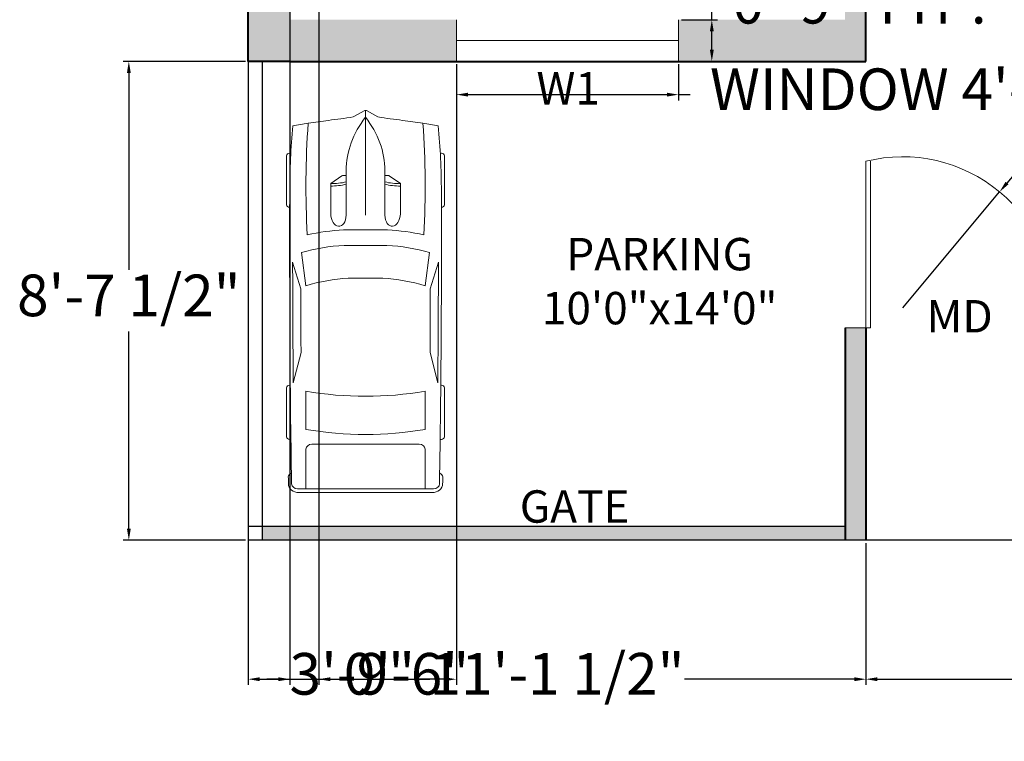
# Model space of a CAD drawing. Units: inches. Extents: x 1883 to 2353, y 1976 to 2541.
# Tile 1 of 5: x 1957 to 2170, y 1976 to 2132. Entities that reach past the tile are written whole.
import ezdxf

# ---------------------------------------------------------------- set-up
doc = ezdxf.new("R2010")
doc.units = ezdxf.units.IN
for name, color, linetype, lineweight in [('A-ANNO-DIMS', 2, 'Continuous', 18), ('A-ANNO-TEXT', 7, 'Continuous', 18), ('A-AREA-IDEN', 7, 'Continuous', 18), ('A-DOOR', 3, 'Continuous', 18), ('A-GLAZ', 4, 'Continuous', 18), ('A-WALL', 7, 'Continuous', 40), ('C-PRKG-VEHI', 8, 'Continuous', 13), ('C-SITE', 7, 'Continuous', 25)]:
    doc.layers.add(name, color=color, linetype=linetype, lineweight=lineweight)
doc.layers.add('A-WALL-PATT', color=67, linetype='Continuous', lineweight=13, true_color=0x727430)
doc.layers.add('C-SITE-PATT', color=18, linetype='Continuous', lineweight=13, true_color=0x000000)
doc.styles.get("Standard").update_dxf_attribs({"font": 'arial.ttf'})
doc.dimstyles.new('ISO-25', dxfattribs={"dimtxt": 9, "dimasz": 2.5, "dimexe": 1.25, "dimexo": 0.625, "dimgap": 2, "dimtad": 0, "dimtih": 1, "dimtoh": 1, "dimdec": 1, "dimlunit": 4, "dimtxsty": 'Standard', "dimcen": 2.5, "dimadec": 0, "dimazin": 0, "dimtfac": 1, "dimtdec": 1, "dimtmove": 0, "dimatfit": 3, "dimfxl": 1, "dimarcsym": 0})

# ---------------------------------------------------------------- blocks, each defined once
blk = doc.blocks.new('*U14')
for p, q in [((46.55, 38.89), (22.35, 38.89)), ((136.7, 38.89), (160.9, 38.89)), ((21.1, 37.41), (21.1, 36.83)), ((47.8, 37.39), (47.8, 37.41)), ((87.99, 31.87), (74.76, 35.92)), ((134.31, 35.6), (119.29, 31.78)), ((135.45, 37.07), (135.45, 37.41)), ((162.15, 37.41), (162.15, 36.77)), ((70.03, 31.54), (86.41, 29.35)), ((138.42, 29.35), (157.25, 29.35)), ((186.47, 29.35), (167.01, 29.35)), ((186.47, -33.5), (186.47, 33.5)), ((188.4, -32.76), (188.4, 32.76)), ((164.52, 26.39), (164.52, -26.39)), ((32.27, 11.63), (36.13, 17.17)), ((36.13, 17.17), (50.94, 17.17)), ((32.12, 9.51), (32.12, 11.15)), ((58.92, -10.77), (58.92, 10.77)), ((66.55, -10.53), (66.55, 10.53)), ((186.47, -10.53), (186.47, 10.53)), ((3.27, 6.13), (0.1, 0.41)), ((29.77, 9.51), (51.68, 9.51)), ((82.74, 8.5), (82.74, -8.5)), ((0, 0), (51.68, 0)), ((0.1, -0.41), (3.27, -6.13)), ((29.77, -9.51), (51.68, -9.51)), ((32.12, -9.51), (32.12, -11.15)), ((32.27, -11.63), (36.13, -17.17)), ((36.13, -17.17), (50.94, -17.17)), ((86.41, -29.35), (70.03, -31.54)), ((87.99, -31.87), (74.76, -35.92)), ((134.31, -35.6), (119.29, -31.78)), ((157.25, -29.35), (138.42, -29.35)), ((167.01, -29.35), (186.47, -29.35)), ((21.1, -37.41), (21.1, -36.83)), ((47.8, -37.39), (47.8, -37.41)), ((135.45, -37.07), (135.45, -37.41)), ((162.15, -37.41), (162.15, -36.77)), ((46.55, -38.89), (22.35, -38.89)), ((136.7, -38.89), (160.9, -38.89))]:
    blk.add_line(p, q)
for centre, major_axis, ratio, start_param, end_param in [((22.35, 37.41), (0, -1.48), 0.842304, 3.141593, 4.712389), ((46.55, 37.41), (0, 1.48), 0.842304, -1.570796, 0), ((136.7, 37.41), (0, -1.48), 0.842304, 3.141593, 4.712389), ((160.9, 37.41), (0, 1.48), 0.842304, -1.570796, 0), ((266.03, -27.52), (0, 313.31), 0.842304, 1.367076, 1.39176), ((41.19, -490.86), (0, 528.23), 0.842304, 0.00281, 0.075598), ((64.48, -10555.62), (0, 10593.03), 0.842304, -0.013397, 0.002797), ((64.48, -10555.62), (0, -10591.55), 0.842304, 3.133765, 3.140441), ((180.63, 35.84), (0, 2.22), 0.842304, -0.013017, 1.249894), ((64.48, -10556.36), (0, 10595.31), 0.842304, -0.013397, -0.013017), ((183.98, 33.5), (0, -2.96), 0.842304, 1.570796, 3.128196), ((183.98, 32.76), (0, -5.25), 0.842304, 1.570796, 3.128196), ((37.47, -593.96), (0, -623.33), 0.842304, 3.096046, 3.200911), ((135.29, 5.39), (0, 81.77), 0.842304, 1.245306, 1.50788), ((149.6, 2.8), (0, -79.58), 0.842304, 4.372215, 4.640744), ((95.79, -3666.35), (0, -3698.24), 0.842304, 3.134049, 3.144098), ((17.08, 0), (0, 147.02), 0.842304, 4.511394, 4.913384), ((35.91, 0), (0, 147.02), 0.842304, 4.511394, 4.913384), ((167.01, 26.39), (0, 2.96), 0.842304, 0, 1.570796), ((259.18, -27.52), (0, -305.3), 0.842304, 4.528606, 4.561838), ((134.4, 5.39), (0, -89.78), 0.842304, 4.449482, 4.652344), ((-204.49, 52.4), (0, -250.96), 0.842304, 1.385369, 1.434372), ((13.04, 17.01), (0, 27.42), 0.842304, 4.435146, 4.718221), ((14.2, 17.01), (0, 27.42), 0.842304, 4.435146, 4.718221), ((50.79, 13.34), (6.34, -0.36), 0.603834, -1.395552, 1.581315), ((32.75, 11.15), (0, 0.74), 0.842304, 0.879714, 1.570796), ((29.77, -46.66), (0, 56.17), 0.842304, 0, 0.590319), ((0.62, 0), (0, -0.74), 0.842304, 4.131459, 5.293319), ((29.77, 46.66), (0, 56.17), 0.842304, 2.551274, 3.141593), ((-204.49, -52.4), (0, 250.96), 0.842304, -1.434372, -1.385369), ((13.04, -17.01), (0, -27.42), 0.842304, 1.564964, 1.848039), ((14.2, -17.01), (0, -27.42), 0.842304, 1.564964, 1.848039), ((149.6, -2.8), (0, -79.58), 0.842304, -1.499151, -1.230623), ((32.75, -11.15), (0, -0.74), 0.842304, 4.712389, 5.403472), ((134.4, -5.39), (0, -89.78), 0.842304, -1.510751, -1.307889), ((135.29, -5.39), (0, -81.77), 0.842304, -1.50788, -1.245306), ((259.18, 27.52), (0, 305.3), 0.842304, 1.721348, 1.754579), ((266.03, 27.52), (0, 313.31), 0.842304, 1.749832, 1.774517), ((37.47, 593.96), (0, -623.33), 0.842304, -0.059319, 0.045547), ((167.01, -26.39), (0, -2.96), 0.842304, 4.712389, 6.283185), ((95.79, 3666.35), (0, -3698.24), 0.842304, -0.002505, 0.007544), ((183.98, -33.5), (0, 2.96), 0.842304, 3.15499, 4.712389), ((183.98, -32.76), (0, -5.25), 0.842304, 0.013397, 1.570796), ((41.19, 490.86), (0, -528.23), 0.842304, -0.075598, -0.00281), ((22.35, -37.41), (0, 1.48), 0.842304, 1.570796, 3.141593), ((64.48, 10555.62), (0, 10593.03), 0.842304, 3.138796, 3.15499), ((46.55, -37.41), (0, -1.48), 0.842304, 0, 1.570796), ((64.48, 10555.62), (0, -10591.55), 0.842304, 0.001152, 0.007828), ((136.7, -37.41), (0, -1.48), 0.842304, -1.570796, 0), ((160.9, -37.41), (0, 1.48), 0.842304, 3.141593, 4.712389), ((180.63, -35.84), (0, -2.22), 0.842304, -1.249894, 0.013017), ((64.48, 10556.36), (0, 10595.31), 0.842304, 3.15461, 3.15499)]:
    blk.add_ellipse(centre, major_axis=major_axis, ratio=ratio, start_param=start_param, end_param=end_param)
at = {"extrusion": (0, 0, -1)}
blk.add_ellipse((50.79, -13.34), major_axis=(6.34, 0.36), ratio=0.603834, start_param=-1.395552, end_param=1.581315, dxfattribs=at)
blk = doc.blocks.new('WIN-48IN')
for p, q in [((0, 0), (0, 9)), ((48, 0), (48, 9)), ((0, 4.5), (48, 4.5))]:
    blk.add_line(p, q)
blk = doc.blocks.new('*D21')
at = {"layer": 'A-ANNO-DIMS', "color": 0, "lineweight": -2, "transparency": 16777216}
for p, q in [((2051.49, 2121.95), (2051.49, 2114.12)), ((2099.49, 2121.95), (2099.49, 2114.12)), ((2053.99, 2115.37), (2096.99, 2115.37)), ((2099.49, 2115.37), (2101.99, 2115.37))]:
    blk.add_line(p, q, dxfattribs=at)
at = {"layer": 'A-ANNO-DIMS', "color": 0, "transparency": 16777216}
for points in [[(2053.99, 2115.79), (2053.99, 2114.96), (2051.49, 2115.37)], [(2096.99, 2115.79), (2096.99, 2114.96), (2099.49, 2115.37)]]:
    blk.add_solid(points, dxfattribs=at)
at = {"layer": 'Defpoints', "color": 0, "transparency": 16777216}
for p in [(2051.49, 2122.57), (2099.49, 2122.57), (2099.49, 2115.37)]:
    blk.add_point(p, dxfattribs=at)
at = {"layer": 'A-ANNO-DIMS', "color": 0, "transparency": 16777216, "insert": (2160.94, 2115.37), "char_height": 9, "attachment_point": 5}
blk.add_mtext('WINDOW 4\'-0" TYP.', dxfattribs=at)
blk = doc.blocks.new('*D22')
at = {"layer": 'A-ANNO-DIMS', "color": 0, "lineweight": -2, "transparency": 16777216}
for p, q in [((2106.69, 2131.57), (2106.69, 2134.07)), ((2106.69, 2134.07), (2109.19, 2134.07)), ((2100.12, 2131.57), (2107.94, 2131.57)), ((2106.69, 2125.07), (2106.69, 2129.07)), ((2100.12, 2122.57), (2107.94, 2122.57))]:
    blk.add_line(p, q, dxfattribs=at)
at = {"layer": 'A-ANNO-DIMS', "color": 0, "transparency": 16777216}
for points in [[(2106.28, 2129.07), (2107.11, 2129.07), (2106.69, 2131.57)], [(2106.28, 2125.07), (2107.11, 2125.07), (2106.69, 2122.57)]]:
    blk.add_solid(points, dxfattribs=at)
at = {"layer": 'Defpoints', "color": 0, "transparency": 16777216}
for p in [(2099.49, 2131.57), (2106.69, 2131.57), (2099.49, 2122.57)]:
    blk.add_point(p, dxfattribs=at)
at = {"layer": 'A-ANNO-DIMS', "color": 0, "transparency": 16777216, "insert": (2138.62, 2134.07), "char_height": 9, "attachment_point": 5}
blk.add_mtext('0\'-9" TYP.', dxfattribs=at)
blk = doc.blocks.new('*D44')
at = {"layer": 'A-ANNO-DIMS', "color": 0, "lineweight": -2, "transparency": 16777216}
for p, q in [((2005.87, 2122.57), (1979.44, 2122.57)), ((1980.69, 2120.07), (1980.69, 2077.48)), ((1980.69, 2021.57), (1980.69, 2064.17)), ((2005.87, 2019.07), (1979.44, 2019.07))]:
    blk.add_line(p, q, dxfattribs=at)
at = {"layer": 'A-ANNO-DIMS', "color": 0, "transparency": 16777216}
for points in [[(1980.28, 2120.07), (1981.11, 2120.07), (1980.69, 2122.57)], [(1980.28, 2021.57), (1981.11, 2021.57), (1980.69, 2019.07)]]:
    blk.add_solid(points, dxfattribs=at)
at = {"layer": 'Defpoints', "color": 0, "transparency": 16777216}
for p in [(1980.69, 2122.57), (2006.49, 2122.57), (2006.49, 2019.07)]:
    blk.add_point(p, dxfattribs=at)
at = {"layer": 'A-ANNO-DIMS', "color": 0, "transparency": 16777216, "insert": (1980.69, 2070.82), "char_height": 9, "attachment_point": 5}
blk.add_mtext('8\'-7 1/2"', dxfattribs=at)
blk = doc.blocks.new('*D45')
at = {"layer": 'A-ANNO-DIMS', "color": 0, "lineweight": -2, "transparency": 16777216}
for p, q in [((2139.99, 2018.45), (2139.99, 1987.78)), ((2180.49, 2018.45), (2180.49, 1987.78)), ((2142.49, 1989.03), (2177.99, 1989.03)), ((2180.49, 1989.03), (2182.99, 1989.03))]:
    blk.add_line(p, q, dxfattribs=at)
at = {"layer": 'A-ANNO-DIMS', "color": 0, "transparency": 16777216}
for points in [[(2142.49, 1989.45), (2142.49, 1988.61), (2139.99, 1989.03)], [(2177.99, 1989.45), (2177.99, 1988.61), (2180.49, 1989.03)]]:
    blk.add_solid(points, dxfattribs=at)
at = {"layer": 'Defpoints', "color": 0, "transparency": 16777216}
for p in [(2139.99, 2019.07), (2180.49, 2019.07), (2180.49, 1989.03)]:
    blk.add_point(p, dxfattribs=at)
at = {"layer": 'A-ANNO-DIMS', "color": 0, "transparency": 16777216, "insert": (2207.44, 1989.03), "char_height": 9, "attachment_point": 5}
blk.add_mtext('3\'-4 1/2"', dxfattribs=at)
blk = doc.blocks.new('*D46')
at = {"layer": 'A-ANNO-DIMS', "color": 0, "lineweight": -2, "transparency": 16777216}
for p, q in [((2006.49, 2018.45), (2006.49, 1987.78)), ((2139.99, 2018.45), (2139.99, 1987.78)), ((2008.99, 1989.03), (2045.72, 1989.03)), ((2137.49, 1989.03), (2100.76, 1989.03))]:
    blk.add_line(p, q, dxfattribs=at)
at = {"layer": 'A-ANNO-DIMS', "color": 0, "transparency": 16777216}
for points in [[(2008.99, 1989.45), (2008.99, 1988.61), (2006.49, 1989.03)], [(2137.49, 1989.45), (2137.49, 1988.61), (2139.99, 1989.03)]]:
    blk.add_solid(points, dxfattribs=at)
at = {"layer": 'Defpoints', "color": 0, "transparency": 16777216}
for p in [(2006.49, 2019.07), (2139.99, 2019.07), (2139.99, 1989.03)]:
    blk.add_point(p, dxfattribs=at)
at = {"layer": 'A-ANNO-DIMS', "color": 0, "transparency": 16777216, "insert": (2073.24, 1989.03), "char_height": 9, "attachment_point": 5}
blk.add_mtext('11\'-1 1/2"', dxfattribs=at)
blk = doc.blocks.new('*D51')
at = {"layer": 'A-ANNO-DIMS', "color": 0, "lineweight": -2, "transparency": 16777216}
for p, q in [((2006.49, 2121.95), (2006.49, 1987.78)), ((2051.49, 2121.95), (2051.49, 1987.78)), ((2008.99, 1989.03), (2015.03, 1989.03)), ((2048.99, 1989.03), (2042.95, 1989.03))]:
    blk.add_line(p, q, dxfattribs=at)
at = {"layer": 'A-ANNO-DIMS', "color": 0, "transparency": 16777216}
for points in [[(2008.99, 1989.45), (2008.99, 1988.61), (2006.49, 1989.03)], [(2048.99, 1989.45), (2048.99, 1988.61), (2051.49, 1989.03)]]:
    blk.add_solid(points, dxfattribs=at)
at = {"layer": 'Defpoints', "color": 0, "transparency": 16777216}
for p in [(2006.49, 2122.57), (2051.49, 2122.57), (2051.49, 1989.03)]:
    blk.add_point(p, dxfattribs=at)
at = {"layer": 'A-ANNO-DIMS', "color": 0, "transparency": 16777216, "insert": (2028.99, 1989.03), "char_height": 9, "attachment_point": 5}
blk.add_mtext('3\'-9"', dxfattribs=at)
blk = doc.blocks.new('*D57')
at = {"layer": 'A-ANNO-DIMS', "color": 0, "lineweight": -2, "transparency": 16777216}
for p, q in [((2015.49, 2307.95), (2015.49, 1987.78)), ((2021.73, 2308.43), (2021.73, 1987.78)), ((2012.99, 1989.03), (2010.49, 1989.03)), ((2015.49, 1989.03), (2021.73, 1989.03)), ((2024.23, 1989.03), (2026.73, 1989.03))]:
    blk.add_line(p, q, dxfattribs=at)
at = {"layer": 'A-ANNO-DIMS', "color": 0, "transparency": 16777216}
for points in [[(2012.99, 1989.45), (2012.99, 1988.61), (2015.49, 1989.03)], [(2024.23, 1989.45), (2024.23, 1988.61), (2021.73, 1989.03)]]:
    blk.add_solid(points, dxfattribs=at)
at = {"layer": 'Defpoints', "color": 0, "transparency": 16777216}
for p in [(2021.73, 2309.06), (2015.49, 2308.57), (2021.73, 1989.03)]:
    blk.add_point(p, dxfattribs=at)
at = {"layer": 'A-ANNO-DIMS', "color": 0, "transparency": 16777216, "insert": (2040.7, 1989.03), "char_height": 9, "attachment_point": 5}
blk.add_mtext('0\'-6"', dxfattribs=at)
blk = doc.blocks.new('*D61')
at = {"layer": 'A-ANNO-DIMS', "color": 0, "lineweight": -2, "transparency": 16777216}
for p, q in [((2181.45, 2109.35), (2170.49, 2096.26)), ((2183.95, 2109.35), (2181.45, 2109.35)), ((2147.95, 2069.32), (2168.88, 2094.34))]:
    blk.add_line(p, q, dxfattribs=at)
at = {"layer": 'A-ANNO-DIMS', "color": 0, "transparency": 16777216}
blk.add_solid([(2170.17, 2096.53), (2170.81, 2095.99), (2168.88, 2094.34)], dxfattribs=at)
at = {"layer": 'Defpoints', "color": 0, "transparency": 16777216}
for p in [(2168.88, 2094.34), (2147.95, 2069.32)]:
    blk.add_point(p, dxfattribs=at)
at = {"layer": 'A-ANNO-DIMS', "color": 0, "transparency": 16777216, "insert": (2212.7, 2109.35), "char_height": 9, "attachment_point": 5}
blk.add_mtext('R2\'-8 1/2"', dxfattribs=at)

msp = doc.modelspace()

# ---------------------------------------------------------------- hatches: boundary and pattern name
at = {"layer": 'A-WALL-PATT'}
h = msp.add_hatch(color=256, dxfattribs=at)
h.dxf.hatch_style = 1
h.paths.add_polyline_path([(2057.49, 2502.07), (2006.49, 2502.07), (2006.49, 2344.57), (2015.49, 2344.57), (2015.49, 2356.57), (2099.49, 2356.57), (2099.49, 2347.93), (2103.99, 2347.93), (2103.99, 2356.57), (2108.06, 2356.57, -0.029386), (2108.06, 2361.07), (2015.49, 2361.07), (2015.49, 2493.07), (2057.49, 2493.07)])
h.paths.add_polyline_path([(2182.74, 2502.07), (2105.49, 2502.07), (2105.49, 2493.07), (2147.49, 2493.07), (2147.49, 2361.07), (2144.06, 2361.07), (2144.06, 2356.57), (2151.99, 2356.57), (2155, 2356.57), (2155, 2361.07), (2151.99, 2361.07), (2151.99, 2493.07), (2182.74, 2493.07)])
h.paths.add_polyline_path([(2270.49, 2502.07), (2230.74, 2502.07), (2230.74, 2493.07), (2261.49, 2493.07), (2261.49, 2361.07), (2191, 2361.07, -0.029386), (2191, 2356.57), (2261.49, 2356.57), (2261.49, 2315.69), (2270.49, 2315.69)])
h.paths.add_polyline_path([(2051.49, 2131.57), (2015.49, 2131.57), (2015.49, 2251.57), (2103.99, 2251.57), (2104.81, 2251.57, -0.028441), (2104.81, 2256.07), (2103.99, 2256.07), (2103.99, 2260.88), (2099.49, 2260.88), (2099.49, 2256.07), (2015.49, 2256.07), (2015.49, 2268.07), (2006.49, 2268.07), (2006.49, 2122.57), (2015.49, 2122.57), (2051.49, 2122.57)])
h.paths.add_polyline_path([(2103.99, 2308.57), (2103.99, 2317.93, -0.034841), (2099.49, 2317.93), (2099.49, 2308.57), (2015.49, 2308.57), (2015.49, 2320.57), (2006.49, 2320.57), (2006.49, 2292.07), (2015.49, 2292.07), (2015.49, 2304.07), (2099.49, 2304.07), (2099.49, 2290.88, -0.034841), (2103.99, 2290.88), (2103.99, 2304.07)])
h = msp.add_hatch(color=256, dxfattribs=at)
h.dxf.hatch_style = 1
h.paths.add_polyline_path([(2189.49, 2090.74), (2180.49, 2090.74), (2180.49, 2071.57, -0.034524), (2180.49, 2067.07), (2189.49, 2067.07), (2261.49, 2067.07), (2270.49, 2067.07), (2270.49, 2094.07), (2270.49, 2255.69), (2261.49, 2255.69), (2261.49, 2200.57), (2261.49, 2196.07), (2261.49, 2094.07), (2261.49, 2076.07), (2189.49, 2076.07)])
h.paths.add_polyline_path([(2189.49, 2196.07), (2208.94, 2196.07), (2208.94, 2200.57), (2151.99, 2200.57), (2139.99, 2200.57), (2139.99, 2251.57), (2139.99, 2256.07), (2135.49, 2256.07), (2134.13, 2256.07), (2134.13, 2251.57), (2135.49, 2251.57), (2135.49, 2131.57), (2099.49, 2131.57), (2099.49, 2122.57), (2103.99, 2122.57), (2135.49, 2122.57), (2139.99, 2122.57), (2139.99, 2196.07), (2151.99, 2196.07), (2180.49, 2196.07), (2180.49, 2136.51), (2189.49, 2136.51)])
h = msp.add_hatch(color=256, dxfattribs=at)
h.dxf.hatch_style = 1
h.paths.add_polyline_path([(2139.99, 2064.96), (2135.49, 2064.96), (2135.49, 2019.07), (2139.99, 2019.07)])
at = {"layer": 'C-SITE-PATT'}
h = msp.add_hatch(color=256, dxfattribs=at)
h.dxf.hatch_style = 1
h.paths.add_polyline_path([(2135.49, 2022.07), (2009.49, 2022.07), (2009.49, 2019.07), (2135.49, 2019.07)])

# ---------------------------------------------------------------- linework, layer by layer
at = {"layer": 'A-DOOR'}
for p, q in [((2139.99, 2064.96), (2139.99, 2100.96)), ((2140.99, 2064.96), (2140.99, 2100.96)), ((2135.49, 2064.96), (2139.99, 2064.96)), ((2140.99, 2064.96), (2139.99, 2064.96))]:
    msp.add_line(p, q, dxfattribs=at)
msp.add_arc((2147.95, 2069.32), 32.63, 356.0455, 104.1079, dxfattribs=at)
at = {"layer": 'A-WALL'}
for p, q in [((2006.49, 2122.57), (2006.49, 2502.07)), ((2139.99, 2122.57), (2139.99, 2196.07)), ((2015.49, 2122.57), (2006.49, 2122.57)), ((2015.49, 2122.57), (2103.99, 2122.57)), ((2103.99, 2122.57), (2135.49, 2122.57)), ((2135.49, 2122.57), (2139.99, 2122.57)), ((2135.49, 2064.96), (2135.49, 2019.07)), ((2139.99, 2064.96), (2139.99, 2019.07))]:
    msp.add_line(p, q, dxfattribs=at)
at = {"layer": 'C-SITE'}
for p, q in [((2006.49, 2122.57), (2006.49, 2019.07)), ((2009.49, 2122.57), (2009.49, 2019.07)), ((2135.49, 2022.07), (2006.49, 2022.07)), ((2180.49, 2019.07), (2006.49, 2019.07))]:
    msp.add_line(p, q, dxfattribs=at)

# ---------------------------------------------------------------- block references
at = {"layer": 'A-GLAZ'}
msp.add_blockref('WIN-48IN', (2051.49, 2122.57), dxfattribs=at)
at = {"layer": 'C-PRKG-VEHI', "xscale": 0.4385878682059836, "yscale": 0.4385878682059836, "zscale": 0.4385878682059836, "rotation": 270}
msp.add_blockref('*U14', (2031.85, 2111.98), dxfattribs=at)

# ---------------------------------------------------------------- texts
at = {"layer": 'A-ANNO-TEXT', "char_height": 7, "attachment_point": 1}
for s, width, insert in [('\\pxqc;{\\fArial|b1|i0|c0|p34;W1}', 23.5361, (2063.88, 2120.24)), ('\\pxqc;{\\fArial|b1|i0|c0|p34;MD}', 14.2427, (2153.13, 2070.98)), ('\\pxqc;{\\fArial|b1|i0|c0|p34;GATE}', 32.08, (2061.01, 2029.86))]:
    msp.add_mtext_dynamic_manual_height_columns(s, width=width, gutter_width=12.5, heights=[0], dxfattribs=dict(at, insert=insert))
at = {"layer": 'A-AREA-IDEN', "insert": (2063.34, 2084.4), "char_height": 7, "attachment_point": 1}
msp.add_mtext_dynamic_manual_height_columns('\\pxqc;{\\fArial|b1|i0|c0|p34;PARKING\\P10\'0"x14\'0"}', width=64.1696, gutter_width=12.5, heights=[0], dxfattribs=at)

# ---------------------------------------------------------------- dimensions: what is measured, and where the dimension line sits
at = {"layer": 'A-ANNO-DIMS'}
for base, p1, p2, picture, middle in [((2021.73, 1989.03), (2015.49, 2308.57), (2021.73, 2309.06), '*D57', (2040.7, 1989.03)), ((2051.49, 1989.03), (2006.49, 2122.57), (2051.49, 2122.57), '*D51', (2028.99, 1989.03)), ((2139.99, 1989.03), (2006.49, 2019.07), (2139.99, 2019.07), '*D46', (2073.24, 1989.03)), ((2180.49, 1989.03), (2139.99, 2019.07), (2180.49, 2019.07), '*D45', (2207.44, 1989.03))]:
    dim = msp.add_linear_dim(base=base, p1=p1, p2=p2, dimstyle='ISO-25', override={"dimdec": 1, "dimlfac": 1, "dimrnd": 0, "dimzin": 1, "dimdsep": 46, "dimlunit": 4, "dimfrac": 2}, dxfattribs=at)
    dim.commit()
    dim.dimension.update_dxf_attribs({"geometry": picture, "text_midpoint": middle})
dim = msp.add_linear_dim(base=(2106.69, 2131.57), p1=(2099.49, 2122.57), p2=(2099.49, 2131.57), angle=90, text='<> TYP.', dimstyle='ISO-25', override={"dimdec": 1, "dimlfac": 1, "dimrnd": 0, "dimzin": 1, "dimdsep": 46, "dimlunit": 4, "dimfrac": 2}, dxfattribs=at)
dim.commit()
dim.dimension.update_dxf_attribs({"geometry": '*D22', "text_midpoint": (2138.62, 2134.07)})
dim = msp.add_linear_dim(base=(2099.49, 2115.37), p1=(2051.49, 2122.57), p2=(2099.49, 2122.57), text='WINDOW <> TYP.', dimstyle='ISO-25', override={"dimdec": 1, "dimlfac": 1, "dimrnd": 0, "dimzin": 1, "dimdsep": 46, "dimlunit": 4, "dimfrac": 2}, dxfattribs=at)
dim.commit()
dim.dimension.update_dxf_attribs({"geometry": '*D21', "text_midpoint": (2160.94, 2115.37)})
dim = msp.add_linear_dim(base=(1980.69, 2122.57), p1=(2006.49, 2019.07), p2=(2006.49, 2122.57), angle=90, dimstyle='ISO-25', override={"dimdec": 1, "dimlfac": 1, "dimrnd": 0, "dimzin": 1, "dimdsep": 46, "dimlunit": 4, "dimfrac": 2}, dxfattribs=at)
dim.commit()
dim.dimension.update_dxf_attribs({"geometry": '*D44', "text_midpoint": (1980.69, 2070.82)})
dim = msp.add_radius_dim(center=(2147.95, 2069.32), mpoint=(2168.88, 2094.34), dimstyle='ISO-25', override={"dimdec": 1, "dimlfac": 1, "dimrnd": 0, "dimzin": 1, "dimdsep": 46, "dimlunit": 4, "dimfrac": 2}, dxfattribs=at)
dim.commit()
dim.dimension.update_dxf_attribs({"geometry": '*D61', "text_midpoint": (2212.7, 2109.35), "dimtype": 164})

doc.saveas('drawing.dxf')
